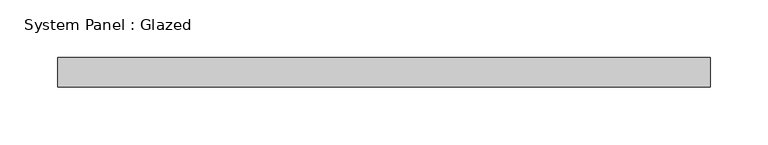
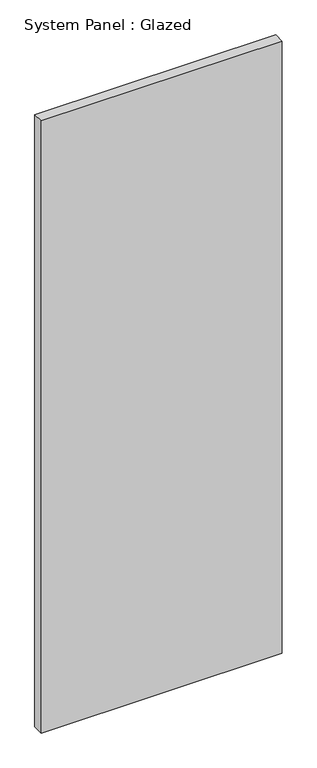
"""IFC4 building model written with IfcOpenShell, lengths in millimetres: plate geometry, System Panel : Glazed."""

from ifc_helpers import new_model, si_unit, origin, origin_with_axes, place, context, project, spatial, polyline, outline, extrude, source, transform, mapped, element, save


def system_panel_glazed_0ced4b38(model_context):
    return source(origin(), model_context, "Body", "SweptSolid", [
        extrude(outline(polyline([(282.575, 19.05), (-282.575, 19.05), (-282.575, 44.45), (282.575, 44.45), (282.575, 19.05)])), origin_with_axes(), (0.0, 0.0, 1.0), 1516.8504197),
    ])


if __name__ == "__main__":
    model = new_model("IFC4")
    model_context = context("Model", 3, world=origin())
    ifc_project = project(units=[si_unit("LENGTHUNIT", "METRE", prefix="MILLI")], contexts=[model_context])
    site = spatial("IfcSite", under=ifc_project)
    building = spatial("IfcBuilding", under=site)
    placement = place(None, origin())
    system_panel_glazed_shape = system_panel_glazed_0ced4b38(model_context)
    element("IfcPlate", 1, ObjectType="System Panel : Glazed", at=placement, inside=building, context=model_context, shape_type="MappedRepresentation", body=[
        mapped(system_panel_glazed_shape, transform((0.0, 0.0, 0.0), x_axis=(1.0, 0.0, 0.0), y_axis=(0.0, 1.0, 0.0), z_axis=(0.0, 0.0, 1.0))),
    ])
    save(model, "model.ifc")

# Revit data of these elements
# Type "System Panel : Glazed"
#   Construction Type Id = "GSP4R"
#   Analytic Construction = "1/8 in Pilkington single glazing"
#   Visual Light Transmittance = 0.9
#   Solar Heat Gain Coefficient = 0.86
#   Heat Transfer Coefficient (U) = 1.18115 BTU/(h·ft²·°F)
#   Define Thermal Properties by = 1
# Element 1 (IfcPlate, "System Panel : Glazed")
#   Materials on its faces: "Glass"
# Materials
#   "Glass": class "Glass", colour RGB 0 128 192, transparency 0.75, Description = "Soda Lime Glass", Cost = 0
